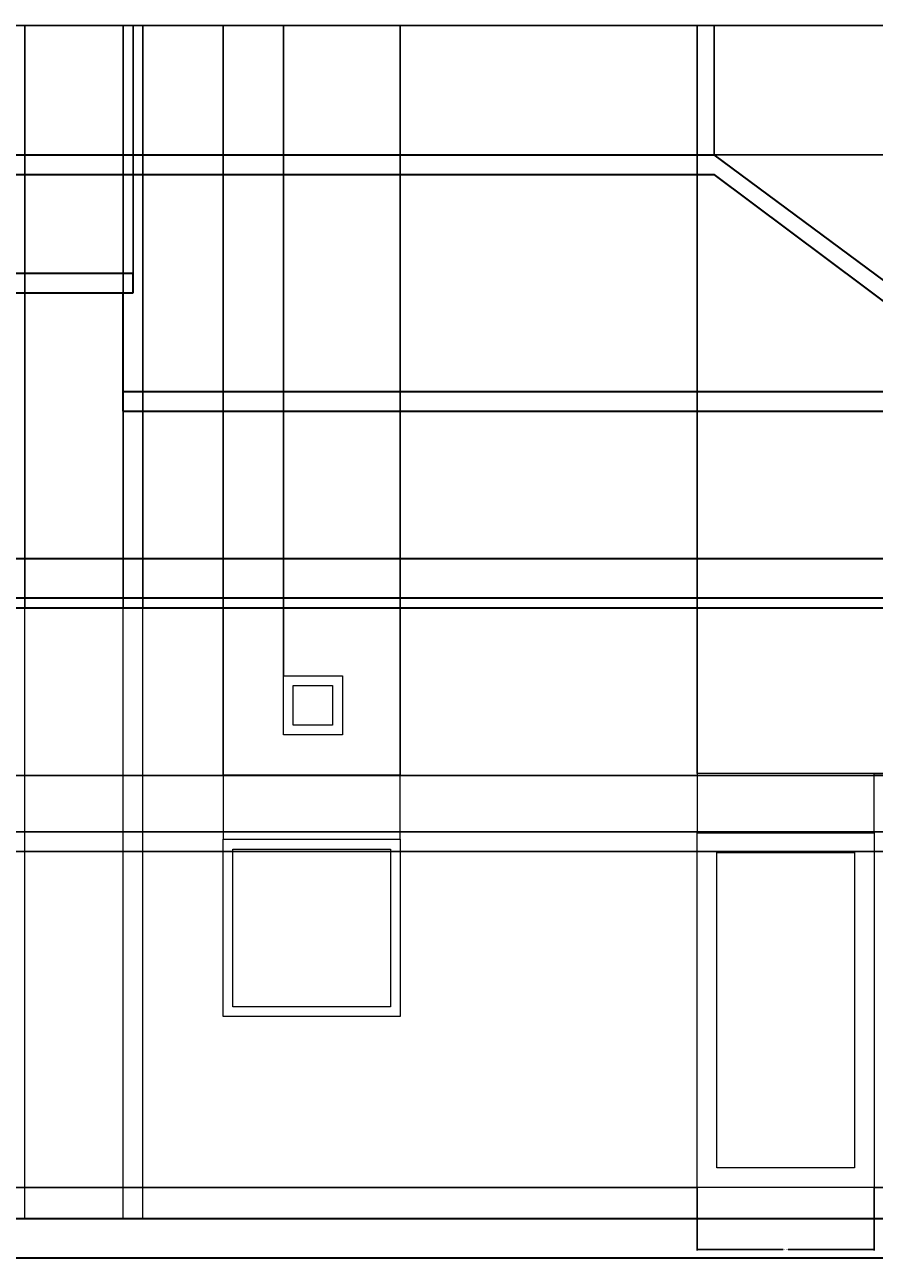
# Model space of a CAD drawing. Units: inches. Extents: x 1817 to 2378, y 1915 to 2370.
# Tile 5 of 8: x 1987 to 2160, y 2119 to 2370. Entities that reach past the tile are written whole.
import ezdxf

# ---------------------------------------------------------------- set-up
doc = ezdxf.new("R2010")
doc.units = ezdxf.units.IN
for name, color, linetype, lineweight in [('A-ANNO-DIMS', 2, 'Continuous', 18), ('A-ELEV', 7, 'Continuous', 35), ('A-GLAZ', 4, 'Continuous', 18), ('P-PIPE', 6, 'Continuous', 18)]:
    doc.layers.add(name, color=color, linetype=linetype, lineweight=lineweight)
doc.styles.get("Standard").update_dxf_attribs({"font": 'arial.ttf'})
doc.dimstyles.get("Standard").update_dxf_attribs({"dimtxt": 0.18, "dimasz": 0.18, "dimexe": 0.18, "dimexo": 0.0625, "dimgap": 0.09, "dimtad": 0, "dimtih": 1, "dimtoh": 1, "dimdec": 4, "dimzin": 0, "dimdsep": 46, "dimtxsty": 'Standard', "dimcen": 0.09, "dimadec": 0, "dimazin": 0, "dimtfac": 1, "dimtdec": 4, "dimtofl": 0, "dimtmove": 0, "dimatfit": 3, "dimfxl": 1, "dimtolj": 1, "dimtzin": 0, "dimarcsym": 0})

# ---------------------------------------------------------------- blocks, each defined once
blk = doc.blocks.new('WIN-SQ-900')
for points in [[(1924.43, 2204.58), (1960.43, 2204.58), (1960.43, 2217.58), (1924.43, 2217.58)], [(1924.43, 2204.58), (1960.43, 2204.58), (1960.43, 2168.58), (1924.43, 2168.58)], [(1926.43, 2202.58), (1958.43, 2202.58), (1958.43, 2170.58), (1926.43, 2170.58)]]:
    blk.add_lwpolyline(points, close=True)
blk = doc.blocks.new('WIN-TALL-900')
for points in [[(2123.62, 2205.9), (2159.62, 2205.9), (2159.62, 2217.9), (2123.62, 2217.9)], [(2123.62, 2205.9), (2159.62, 2205.9), (2159.62, 2133.9), (2123.62, 2133.9)], [(2127.62, 2201.9), (2155.62, 2201.9), (2155.62, 2137.9), (2127.62, 2137.9)]]:
    blk.add_lwpolyline(points, close=True)
blk = doc.blocks.new('VENT-300')
for points in [[(1936.66, 2237.16), (1948.66, 2237.16), (1948.66, 2225.16), (1936.66, 2225.16)], [(1938.66, 2235.16), (1946.66, 2235.16), (1946.66, 2227.16), (1938.66, 2227.16)]]:
    blk.add_lwpolyline(points, close=True)
blk = doc.blocks.new('*D8')
at = {"layer": 'A-ANNO-DIMS', "color": 0, "lineweight": -2, "transparency": 16777216}
for p, q in [((2159.68, 2217.9), (2172.4, 2217.9)), ((2172.22, 2217.72), (2172.22, 2176.08)), ((2172.22, 2134.08), (2172.22, 2175.71)), ((2159.68, 2133.9), (2172.4, 2133.9))]:
    blk.add_line(p, q, dxfattribs=at)
at = {"layer": 'A-ANNO-DIMS', "color": 0, "transparency": 16777216}
for points in [[(2172.19, 2217.72), (2172.25, 2217.72), (2172.22, 2217.9)], [(2172.19, 2134.08), (2172.25, 2134.08), (2172.22, 2133.9)]]:
    blk.add_solid(points, dxfattribs=at)
at = {"layer": 'Defpoints', "color": 0, "transparency": 16777216}
for p in [(2159.62, 2217.9), (2172.22, 2217.9), (2159.62, 2133.9)]:
    blk.add_point(p, dxfattribs=at)
at = {"layer": 'A-ANNO-DIMS', "color": 0, "transparency": 16777216, "insert": (2172.22, 2175.9), "char_height": 0.18, "attachment_point": 5}
blk.add_mtext('\\A1;TALL WINDOW 84 TYP.', dxfattribs=at)
blk = doc.blocks.new('*D9')
at = {"layer": 'A-ANNO-DIMS', "color": 0, "lineweight": -2, "transparency": 16777216}
for p, q in [((2123.62, 2133.83), (2123.62, 2121.12)), ((2159.62, 2133.83), (2159.62, 2121.12)), ((2123.8, 2121.3), (2141.09, 2121.3)), ((2159.44, 2121.3), (2142.15, 2121.3))]:
    blk.add_line(p, q, dxfattribs=at)
at = {"layer": 'A-ANNO-DIMS', "color": 0, "transparency": 16777216}
for points in [[(2123.8, 2121.33), (2123.8, 2121.27), (2123.62, 2121.3)], [(2159.44, 2121.33), (2159.44, 2121.27), (2159.62, 2121.3)]]:
    blk.add_solid(points, dxfattribs=at)
at = {"layer": 'Defpoints', "color": 0, "transparency": 16777216}
for p in [(2123.62, 2133.9), (2159.62, 2133.9), (2159.62, 2121.3)]:
    blk.add_point(p, dxfattribs=at)
at = {"layer": 'A-ANNO-DIMS', "color": 0, "transparency": 16777216, "insert": (2141.62, 2121.3), "char_height": 0.18, "attachment_point": 5}
blk.add_mtext('\\A1;36 TYP.', dxfattribs=at)
blk = doc.blocks.new('*D23')
at = {"layer": 'A-ANNO-DIMS', "color": 0, "lineweight": -2, "transparency": 16777216}
for p, q in [((2320.11, 2156.45), (2320.11, 1915.08)), ((1867.08, 1965.45), (1867.08, 1915.08)), ((1867.26, 1915.26), (2093.3, 1915.26)), ((2319.93, 1915.26), (2093.89, 1915.26))]:
    blk.add_line(p, q, dxfattribs=at)
at = {"layer": 'A-ANNO-DIMS', "color": 0, "transparency": 16777216}
for points in [[(1867.26, 1915.29), (1867.26, 1915.23), (1867.08, 1915.26)], [(2319.93, 1915.29), (2319.93, 1915.23), (2320.11, 1915.26)]]:
    blk.add_solid(points, dxfattribs=at)
at = {"layer": 'Defpoints', "color": 0, "transparency": 16777216}
for p in [(2320.11, 2156.51), (1867.08, 1965.51), (2320.11, 1915.26)]:
    blk.add_point(p, dxfattribs=at)
at = {"layer": 'A-ANNO-DIMS', "color": 0, "transparency": 16777216, "insert": (2093.6, 1915.26), "char_height": 0.18, "attachment_point": 5}
blk.add_mtext('\\A1;453', dxfattribs=at)
blk = doc.blocks.new('*D30')
at = {"layer": 'A-ANNO-DIMS', "color": 0, "lineweight": -2, "transparency": 16777216}
for p, q in [((1987.08, 2251.57), (1987.08, 2369.94)), ((1987.26, 2369.76), (1996.86, 2369.76)), ((2006.9, 2369.76), (1997.31, 2369.76)), ((2007.08, 2251.57), (2007.08, 2369.94))]:
    blk.add_line(p, q, dxfattribs=at)
at = {"layer": 'A-ANNO-DIMS', "color": 0, "transparency": 16777216}
for points in [[(1987.26, 2369.79), (1987.26, 2369.73), (1987.08, 2369.76)], [(2006.9, 2369.79), (2006.9, 2369.73), (2007.08, 2369.76)]]:
    blk.add_solid(points, dxfattribs=at)
at = {"layer": 'Defpoints', "color": 0, "transparency": 16777216}
for p in [(2007.08, 2369.76), (1987.08, 2251.51), (2007.08, 2251.51)]:
    blk.add_point(p, dxfattribs=at)
at = {"layer": 'A-ANNO-DIMS', "color": 0, "transparency": 16777216, "insert": (1997.08, 2369.76), "char_height": 0.18, "attachment_point": 5}
blk.add_mtext('\\A1;20', dxfattribs=at)
blk = doc.blocks.new('*D31')
at = {"layer": 'A-ANNO-DIMS', "color": 0, "lineweight": -2, "transparency": 16777216}
for p, q in [((2007.08, 2251.57), (2007.08, 2369.94)), ((2007.26, 2369.76), (2008.93, 2369.76)), ((2010.9, 2369.76), (2009.24, 2369.76)), ((2011.08, 2251.57), (2011.08, 2369.94))]:
    blk.add_line(p, q, dxfattribs=at)
at = {"layer": 'A-ANNO-DIMS', "color": 0, "transparency": 16777216}
for points in [[(2007.26, 2369.79), (2007.26, 2369.73), (2007.08, 2369.76)], [(2010.9, 2369.79), (2010.9, 2369.73), (2011.08, 2369.76)]]:
    blk.add_solid(points, dxfattribs=at)
at = {"layer": 'Defpoints', "color": 0, "transparency": 16777216}
for p in [(2011.08, 2369.76), (2007.08, 2251.51), (2011.08, 2251.51)]:
    blk.add_point(p, dxfattribs=at)
at = {"layer": 'A-ANNO-DIMS', "color": 0, "transparency": 16777216, "insert": (2009.08, 2369.76), "char_height": 0.18, "attachment_point": 5}
blk.add_mtext('\\A1;4', dxfattribs=at)
blk = doc.blocks.new('*D32')
at = {"layer": 'A-ANNO-DIMS', "color": 0, "lineweight": -2, "transparency": 16777216}
for p, q in [((2011.08, 2251.57), (2011.08, 2369.94)), ((2011.26, 2369.76), (2018.83, 2369.76)), ((2027.17, 2369.76), (2019.61, 2369.76)), ((2027.35, 2217.64), (2027.35, 2369.94))]:
    blk.add_line(p, q, dxfattribs=at)
at = {"layer": 'A-ANNO-DIMS', "color": 0, "transparency": 16777216}
for points in [[(2011.26, 2369.79), (2011.26, 2369.73), (2011.08, 2369.76)], [(2027.17, 2369.79), (2027.17, 2369.73), (2027.35, 2369.76)]]:
    blk.add_solid(points, dxfattribs=at)
at = {"layer": 'Defpoints', "color": 0, "transparency": 16777216}
for p in [(2027.35, 2369.76), (2011.08, 2251.51), (2027.35, 2217.58)]:
    blk.add_point(p, dxfattribs=at)
at = {"layer": 'A-ANNO-DIMS', "color": 0, "transparency": 16777216, "insert": (2019.22, 2369.76), "char_height": 0.18, "attachment_point": 5}
blk.add_mtext('\\A1;16.27', dxfattribs=at)
blk = doc.blocks.new('*D33')
at = {"layer": 'A-ANNO-DIMS', "color": 0, "lineweight": -2, "transparency": 16777216}
for p, q in [((2027.35, 2217.64), (2027.35, 2369.94)), ((2027.53, 2369.76), (2033.03, 2369.76)), ((2039.43, 2369.76), (2033.94, 2369.76)), ((2039.61, 2237.83), (2039.61, 2369.94))]:
    blk.add_line(p, q, dxfattribs=at)
at = {"layer": 'A-ANNO-DIMS', "color": 0, "transparency": 16777216}
for points in [[(2027.53, 2369.79), (2027.53, 2369.73), (2027.35, 2369.76)], [(2039.43, 2369.79), (2039.43, 2369.73), (2039.61, 2369.76)]]:
    blk.add_solid(points, dxfattribs=at)
at = {"layer": 'Defpoints', "color": 0, "transparency": 16777216}
for p in [(2039.61, 2369.76), (2039.61, 2237.77), (2027.35, 2217.58)]:
    blk.add_point(p, dxfattribs=at)
at = {"layer": 'A-ANNO-DIMS', "color": 0, "transparency": 16777216, "insert": (2033.48, 2369.76), "char_height": 0.18, "attachment_point": 5}
blk.add_mtext('\\A1;12.256', dxfattribs=at)
blk = doc.blocks.new('*D34')
at = {"layer": 'A-ANNO-DIMS', "color": 0, "lineweight": -2, "transparency": 16777216}
for p, q in [((2039.61, 2237.83), (2039.61, 2369.94)), ((2039.79, 2369.76), (2051.02, 2369.76)), ((2063.17, 2369.76), (2051.95, 2369.76)), ((2063.35, 2217.64), (2063.35, 2369.94))]:
    blk.add_line(p, q, dxfattribs=at)
at = {"layer": 'A-ANNO-DIMS', "color": 0, "transparency": 16777216}
for points in [[(2039.79, 2369.79), (2039.79, 2369.73), (2039.61, 2369.76)], [(2063.17, 2369.79), (2063.17, 2369.73), (2063.35, 2369.76)]]:
    blk.add_solid(points, dxfattribs=at)
at = {"layer": 'Defpoints', "color": 0, "transparency": 16777216}
for p in [(2063.35, 2369.76), (2039.61, 2237.77), (2063.35, 2217.58)]:
    blk.add_point(p, dxfattribs=at)
at = {"layer": 'A-ANNO-DIMS', "color": 0, "transparency": 16777216, "insert": (2051.48, 2369.76), "char_height": 0.18, "attachment_point": 5}
blk.add_mtext('\\A1;23.744', dxfattribs=at)
blk = doc.blocks.new('*D35')
at = {"layer": 'A-ANNO-DIMS', "color": 0, "lineweight": -2, "transparency": 16777216}
for p, q in [((2063.35, 2217.64), (2063.35, 2369.94)), ((2063.53, 2369.76), (2093.09, 2369.76)), ((2123.44, 2369.76), (2093.88, 2369.76)), ((2123.62, 2217.96), (2123.62, 2369.94))]:
    blk.add_line(p, q, dxfattribs=at)
at = {"layer": 'A-ANNO-DIMS', "color": 0, "transparency": 16777216}
for points in [[(2063.53, 2369.79), (2063.53, 2369.73), (2063.35, 2369.76)], [(2123.44, 2369.79), (2123.44, 2369.73), (2123.62, 2369.76)]]:
    blk.add_solid(points, dxfattribs=at)
at = {"layer": 'Defpoints', "color": 0, "transparency": 16777216}
for p in [(2123.62, 2369.76), (2123.62, 2217.9), (2063.35, 2217.58)]:
    blk.add_point(p, dxfattribs=at)
at = {"layer": 'A-ANNO-DIMS', "color": 0, "transparency": 16777216, "insert": (2093.49, 2369.76), "char_height": 0.18, "attachment_point": 5}
blk.add_mtext('\\A1;60.26', dxfattribs=at)
blk = doc.blocks.new('*D44')
at = {"layer": 'A-ANNO-DIMS', "color": 0, "lineweight": -2, "transparency": 16777216}
for p, q in [((1903.08, 2261.57), (1903.08, 2369.94)), ((1903.26, 2369.76), (1954.8, 2369.76)), ((2006.9, 2369.76), (1955.36, 2369.76)), ((2007.08, 2291.57), (2007.08, 2369.94))]:
    blk.add_line(p, q, dxfattribs=at)
at = {"layer": 'A-ANNO-DIMS', "color": 0, "transparency": 16777216}
for points in [[(1903.26, 2369.79), (1903.26, 2369.73), (1903.08, 2369.76)], [(2006.9, 2369.79), (2006.9, 2369.73), (2007.08, 2369.76)]]:
    blk.add_solid(points, dxfattribs=at)
at = {"layer": 'Defpoints', "color": 0, "transparency": 16777216}
for p in [(2007.08, 2369.76), (2007.08, 2291.51), (1903.08, 2261.51)]:
    blk.add_point(p, dxfattribs=at)
at = {"layer": 'A-ANNO-DIMS', "color": 0, "transparency": 16777216, "insert": (1955.08, 2369.76), "char_height": 0.18, "attachment_point": 5}
blk.add_mtext('\\A1;104', dxfattribs=at)
blk = doc.blocks.new('*D45')
at = {"layer": 'A-ANNO-DIMS', "color": 0, "lineweight": -2, "transparency": 16777216}
for p, q in [((2007.08, 2291.57), (2007.08, 2369.94)), ((2007.26, 2369.76), (2007.94, 2369.76)), ((2008.9, 2369.76), (2008.23, 2369.76)), ((2009.08, 2319.57), (2009.08, 2369.94))]:
    blk.add_line(p, q, dxfattribs=at)
at = {"layer": 'A-ANNO-DIMS', "color": 0, "transparency": 16777216}
for points in [[(2007.26, 2369.79), (2007.26, 2369.73), (2007.08, 2369.76)], [(2008.9, 2369.79), (2008.9, 2369.73), (2009.08, 2369.76)]]:
    blk.add_solid(points, dxfattribs=at)
at = {"layer": 'Defpoints', "color": 0, "transparency": 16777216}
for p in [(2009.08, 2369.76), (2009.08, 2319.51), (2007.08, 2291.51)]:
    blk.add_point(p, dxfattribs=at)
at = {"layer": 'A-ANNO-DIMS', "color": 0, "transparency": 16777216, "insert": (2008.08, 2369.76), "char_height": 0.18, "attachment_point": 5}
blk.add_mtext('\\A1;2', dxfattribs=at)
blk = doc.blocks.new('*D46')
at = {"layer": 'A-ANNO-DIMS', "color": 0, "lineweight": -2, "transparency": 16777216}
for p, q in [((2009.08, 2319.57), (2009.08, 2369.94)), ((2009.26, 2369.76), (2067.8, 2369.76)), ((2126.9, 2369.76), (2068.37, 2369.76)), ((2127.08, 2343.57), (2127.08, 2369.94))]:
    blk.add_line(p, q, dxfattribs=at)
at = {"layer": 'A-ANNO-DIMS', "color": 0, "transparency": 16777216}
for points in [[(2009.26, 2369.79), (2009.26, 2369.73), (2009.08, 2369.76)], [(2126.9, 2369.79), (2126.9, 2369.73), (2127.08, 2369.76)]]:
    blk.add_solid(points, dxfattribs=at)
at = {"layer": 'Defpoints', "color": 0, "transparency": 16777216}
for p in [(2127.08, 2369.76), (2127.08, 2343.51), (2009.08, 2319.51)]:
    blk.add_point(p, dxfattribs=at)
at = {"layer": 'A-ANNO-DIMS', "color": 0, "transparency": 16777216, "insert": (2068.08, 2369.76), "char_height": 0.18, "attachment_point": 5}
blk.add_mtext('\\A1;118', dxfattribs=at)
blk = doc.blocks.new('*D47')
at = {"layer": 'A-ANNO-DIMS', "color": 0, "lineweight": -2, "transparency": 16777216}
for p, q in [((2127.08, 2343.57), (2127.08, 2369.94)), ((2127.26, 2369.76), (2159.09, 2369.76)), ((2191.7, 2369.76), (2159.87, 2369.76)), ((2191.88, 2295.57), (2191.88, 2369.94))]:
    blk.add_line(p, q, dxfattribs=at)
at = {"layer": 'A-ANNO-DIMS', "color": 0, "transparency": 16777216}
for points in [[(2127.26, 2369.79), (2127.26, 2369.73), (2127.08, 2369.76)], [(2191.7, 2369.79), (2191.7, 2369.73), (2191.88, 2369.76)]]:
    blk.add_solid(points, dxfattribs=at)
at = {"layer": 'Defpoints', "color": 0, "transparency": 16777216}
for p in [(2191.88, 2369.76), (2127.08, 2343.51), (2191.88, 2295.51)]:
    blk.add_point(p, dxfattribs=at)
at = {"layer": 'A-ANNO-DIMS', "color": 0, "transparency": 16777216, "insert": (2159.48, 2369.76), "char_height": 0.18, "attachment_point": 5}
blk.add_mtext('\\A1;64.79', dxfattribs=at)
blk = doc.blocks.new('*D51')
at = {"layer": 'A-ANNO-DIMS', "color": 0, "lineweight": -2, "transparency": 16777216}
for p, q in [((2281.02, 2261.51), (1817.4, 2261.51)), ((1817.58, 2261.33), (1817.58, 2257.69)), ((1817.58, 2253.69), (1817.58, 2257.33)), ((2289.54, 2253.51), (1817.4, 2253.51))]:
    blk.add_line(p, q, dxfattribs=at)
at = {"layer": 'A-ANNO-DIMS', "color": 0, "transparency": 16777216}
for points in [[(1817.55, 2261.33), (1817.61, 2261.33), (1817.58, 2261.51)], [(1817.55, 2253.69), (1817.61, 2253.69), (1817.58, 2253.51)]]:
    blk.add_solid(points, dxfattribs=at)
at = {"layer": 'Defpoints', "color": 0, "transparency": 16777216}
for p in [(1817.58, 2261.51), (2281.08, 2261.51), (2289.61, 2253.51)]:
    blk.add_point(p, dxfattribs=at)
at = {"layer": 'A-ANNO-DIMS', "color": 0, "transparency": 16777216, "insert": (1817.58, 2257.51), "char_height": 0.18, "attachment_point": 5}
blk.add_mtext('\\A1;8', dxfattribs=at)
blk = doc.blocks.new('*D79')
at = {"layer": 'A-ANNO-DIMS', "color": 0, "lineweight": -2, "transparency": 16777216}
for p, q in [((2127.15, 2343.51), (2377.4, 2343.51)), ((2377.22, 2343.33), (2377.22, 2319.69)), ((2377.22, 2295.69), (2377.22, 2319.33)), ((2283.15, 2295.51), (2377.4, 2295.51))]:
    blk.add_line(p, q, dxfattribs=at)
at = {"layer": 'A-ANNO-DIMS', "color": 0, "transparency": 16777216}
for points in [[(2377.19, 2343.33), (2377.25, 2343.33), (2377.22, 2343.51)], [(2377.19, 2295.69), (2377.25, 2295.69), (2377.22, 2295.51)]]:
    blk.add_solid(points, dxfattribs=at)
at = {"layer": 'Defpoints', "color": 0, "transparency": 16777216}
for p in [(2127.08, 2343.51), (2377.22, 2343.51), (2283.08, 2295.51)]:
    blk.add_point(p, dxfattribs=at)
at = {"layer": 'A-ANNO-DIMS', "color": 0, "transparency": 16777216, "insert": (2377.22, 2319.51), "char_height": 0.18, "attachment_point": 5}
blk.add_mtext('\\A1;48', dxfattribs=at)
blk = doc.blocks.new('*D82')
at = {"layer": 'A-ANNO-DIMS', "color": 0, "lineweight": -2, "transparency": 16777216}
for p, q in [((2123.56, 2133.9), (1817.4, 2133.9)), ((1817.58, 2133.72), (1817.58, 2130.88)), ((1817.58, 2127.69), (1817.58, 2130.52)), ((2198.53, 2127.51), (1817.4, 2127.51))]:
    blk.add_line(p, q, dxfattribs=at)
at = {"layer": 'A-ANNO-DIMS', "color": 0, "transparency": 16777216}
for points in [[(1817.55, 2133.72), (1817.61, 2133.72), (1817.58, 2133.9)], [(1817.55, 2127.69), (1817.61, 2127.69), (1817.58, 2127.51)]]:
    blk.add_solid(points, dxfattribs=at)
at = {"layer": 'Defpoints', "color": 0, "transparency": 16777216}
for p in [(1817.58, 2133.9), (2123.62, 2133.9), (2198.59, 2127.51)]:
    blk.add_point(p, dxfattribs=at)
at = {"layer": 'A-ANNO-DIMS', "color": 0, "transparency": 16777216, "insert": (1817.58, 2130.7), "char_height": 0.18, "attachment_point": 5}
blk.add_mtext('\\A1;6.387', dxfattribs=at)
blk = doc.blocks.new('*D104')
at = {"layer": 'A-ANNO-DIMS', "color": 0, "lineweight": -2, "transparency": 16777216}
for p, q in [((2210.55, 2217.51), (1817.4, 2217.51)), ((1817.58, 2217.33), (1817.58, 2211.97)), ((1817.58, 2206.26), (1817.58, 2211.61)), ((2210.55, 2206.08), (1817.4, 2206.08))]:
    blk.add_line(p, q, dxfattribs=at)
at = {"layer": 'A-ANNO-DIMS', "color": 0, "transparency": 16777216}
for points in [[(1817.55, 2217.33), (1817.61, 2217.33), (1817.58, 2217.51)], [(1817.55, 2206.26), (1817.61, 2206.26), (1817.58, 2206.08)]]:
    blk.add_solid(points, dxfattribs=at)
at = {"layer": 'Defpoints', "color": 0, "transparency": 16777216}
for p in [(2210.62, 2217.51), (1817.58, 2206.08), (2210.62, 2206.08)]:
    blk.add_point(p, dxfattribs=at)
at = {"layer": 'A-ANNO-DIMS', "color": 0, "transparency": 16777216, "insert": (1817.58, 2211.79), "char_height": 0.18, "attachment_point": 5}
blk.add_mtext('\\A1;11.433', dxfattribs=at)
blk = doc.blocks.new('*D105')
at = {"layer": 'A-ANNO-DIMS', "color": 0, "lineweight": -2, "transparency": 16777216}
for p, q in [((2210.55, 2206.08), (1817.4, 2206.08)), ((1817.58, 2205.9), (1817.58, 2204.26)), ((1817.58, 2202.26), (1817.58, 2203.89)), ((2214.55, 2202.08), (1817.4, 2202.08))]:
    blk.add_line(p, q, dxfattribs=at)
at = {"layer": 'A-ANNO-DIMS', "color": 0, "transparency": 16777216}
for points in [[(1817.55, 2205.9), (1817.61, 2205.9), (1817.58, 2206.08)], [(1817.55, 2202.26), (1817.61, 2202.26), (1817.58, 2202.08)]]:
    blk.add_solid(points, dxfattribs=at)
at = {"layer": 'Defpoints', "color": 0, "transparency": 16777216}
for p in [(2210.62, 2206.08), (1817.58, 2202.08), (2214.62, 2202.08)]:
    blk.add_point(p, dxfattribs=at)
at = {"layer": 'A-ANNO-DIMS', "color": 0, "transparency": 16777216, "insert": (1817.58, 2204.08), "char_height": 0.18, "attachment_point": 5}
blk.add_mtext('\\A1;4.00', dxfattribs=at)
blk = doc.blocks.new('*D119')
at = {"layer": 'A-ANNO-DIMS', "color": 0, "lineweight": -2, "transparency": 16777216}
for p, q in [((1903.08, 1989.57), (1903.08, 2369.94)), ((1903.26, 2369.76), (2091.62, 2369.76)), ((2280.9, 2369.76), (2092.55, 2369.76)), ((2281.08, 1989.57), (2281.08, 2369.94))]:
    blk.add_line(p, q, dxfattribs=at)
at = {"layer": 'A-ANNO-DIMS', "color": 0, "transparency": 16777216}
for points in [[(1903.26, 2369.79), (1903.26, 2369.73), (1903.08, 2369.76)], [(2280.9, 2369.79), (2280.9, 2369.73), (2281.08, 2369.76)]]:
    blk.add_solid(points, dxfattribs=at)
at = {"layer": 'Defpoints', "color": 0, "transparency": 16777216}
for p in [(2281.08, 2369.76), (1903.08, 1989.51), (2281.08, 1989.51)]:
    blk.add_point(p, dxfattribs=at)
at = {"layer": 'A-ANNO-DIMS', "color": 0, "transparency": 16777216, "insert": (2092.08, 2369.76), "char_height": 0.18, "attachment_point": 5}
blk.add_mtext('\\A1;378.00', dxfattribs=at)

msp = doc.modelspace()

# ---------------------------------------------------------------- linework, layer by layer
at = {"layer": 'A-ELEV'}
for p, q in [((1901.0849, 2343.5087), (2127.0849, 2343.5087)), ((2191.8757, 2295.5087), (2127.0849, 2343.5087)), ((1901.0849, 2339.5087), (2127.0849, 2339.5087)), ((2186.0507, 2295.5087), (2127.0849, 2339.5087)), ((1901.0849, 2319.5087), (2009.0849, 2319.5087)), ((2009.0849, 2315.5087), (2009.0849, 2319.5087)), ((1901.0849, 2315.5087), (2009.0849, 2315.5087)), ((2007.0849, 2291.5087), (2007.0849, 2315.5087)), ((2007.0849, 2295.5087), (2283.0849, 2295.5087)), ((2007.0849, 2291.5087), (2283.0849, 2291.5087)), ((2281.0849, 2261.5087), (1903.0849, 2261.5087)), ((2289.6055, 2253.5087), (1894.506, 2253.5087)), ((2289.6055, 2251.5087), (1894.506, 2251.5087)), ((2198.5896, 2127.5087), (1903.0849, 2127.5087)), ((2198.5896, 2119.5087), (1895.6961, 2119.5087))]:
    msp.add_line(p, q, dxfattribs=at)
at = {"layer": 'P-PIPE'}
for p, q in [((1987.0849, 2127.5087), (1987.0849, 2251.5087)), ((2007.0849, 2127.5087), (2007.0849, 2251.5087)), ((2011.0849, 2127.5087), (2011.0849, 2251.5087))]:
    msp.add_line(p, q, dxfattribs=at)

# ---------------------------------------------------------------- block references
at = {"layer": 'A-GLAZ'}
for name, p in [('VENT-300', (102.9456, 0.6122)), ('WIN-TALL-900', (0, 0)), ('WIN-SQ-900', (102.9291, 0))]:
    msp.add_blockref(name, p, dxfattribs=at)

# ---------------------------------------------------------------- dimensions: what is measured, and where the dimension line sits
at = {"layer": 'A-ANNO-DIMS'}
for base, p1, p2, override, picture, middle in [((2007.0849, 2369.7587), (1903.0849, 2261.5087), (2007.0849, 2291.5087), {"dimdec": 0, "dimlfac": 1, "dimrnd": 0, "dimzin": 0, "dimdsep": 46, "dimlunit": 2}, '*D44', (1955.0849, 2369.7587)), ((2281.0849, 2369.7587), (1903.0849, 1989.5087), (2281.0849, 1989.5087), {"dimdec": 2, "dimlfac": 1, "dimrnd": 0, "dimzin": 0, "dimdsep": 46, "dimlunit": 2}, '*D119', (2092.0849, 2369.7587)), ((2007.0849, 2369.7587), (1987.0849, 2251.5087), (2007.0849, 2251.5087), {"dimdec": 0, "dimlfac": 1, "dimrnd": 0, "dimzin": 0, "dimdsep": 46, "dimlunit": 2}, '*D30', (1997.0849, 2369.7587)), ((2011.0849, 2369.7587), (2007.0849, 2251.5087), (2011.0849, 2251.5087), {"dimdec": 0, "dimlfac": 1, "dimrnd": 0, "dimzin": 0, "dimdsep": 46, "dimlunit": 2}, '*D31', (2009.0849, 2369.7587)), ((2009.0849, 2369.7587), (2007.0849, 2291.5087), (2009.0849, 2319.5087), {"dimdec": 0, "dimlfac": 1, "dimrnd": 0, "dimzin": 0, "dimdsep": 46, "dimlunit": 2}, '*D45', (2008.0849, 2369.7587)), ((2127.0849, 2369.7587), (2009.0849, 2319.5087), (2127.0849, 2343.5087), {"dimdec": 0, "dimlfac": 1, "dimrnd": 0, "dimzin": 0, "dimdsep": 46, "dimlunit": 2}, '*D46', (2068.0849, 2369.7587)), ((2027.3548, 2369.7587), (2011.0849, 2251.5087), (2027.3548, 2217.5813), {"dimdec": 2, "dimlfac": 1, "dimrnd": 0, "dimzin": 0, "dimdsep": 46, "dimlunit": 2}, '*D32', (2019.2199, 2369.7587)), ((2039.6105, 2369.7587), (2027.3548, 2217.5813), (2039.6105, 2237.7713), {"dimdec": 3, "dimlfac": 1, "dimrnd": 0, "dimzin": 0, "dimdsep": 46, "dimlunit": 2}, '*D33', (2033.4827, 2369.7587)), ((2063.3548, 2369.7587), (2039.6105, 2237.7713), (2063.3548, 2217.5813), {"dimdec": 3, "dimlfac": 1, "dimrnd": 0, "dimzin": 0, "dimdsep": 46, "dimlunit": 2}, '*D34', (2051.4827, 2369.7587)), ((2123.6179, 2369.7587), (2063.3548, 2217.5813), (2123.6179, 2217.8955), {"dimdec": 2, "dimlfac": 1, "dimrnd": 0, "dimzin": 0, "dimdsep": 46, "dimlunit": 2}, '*D35', (2093.4864, 2369.7587)), ((2191.8757, 2369.7587), (2127.0849, 2343.5087), (2191.8757, 2295.5087), {"dimdec": 2, "dimlfac": 1, "dimrnd": 0, "dimzin": 0, "dimdsep": 46, "dimlunit": 2}, '*D47', (2159.4803, 2369.7587)), ((2320.1054, 1915.2587), (1867.0849, 1965.5087), (2320.1054, 2156.5133), {"dimdec": 0, "dimlfac": 1, "dimrnd": 0, "dimzin": 0, "dimdsep": 46, "dimlunit": 2}, '*D23', (2093.5951, 1915.2587))]:
    dim = msp.add_linear_dim(base=base, p1=p1, p2=p2, dimstyle='Standard', override=override, dxfattribs=at)
    dim.commit()
    dim.dimension.update_dxf_attribs({"geometry": picture, "text_midpoint": middle})
for base, p1, p2, override, picture, middle in [((2377.2181, 2343.5087), (2283.0849, 2295.5087), (2127.0849, 2343.5087), {"dimdec": 0, "dimlfac": 1, "dimrnd": 0, "dimzin": 0, "dimdsep": 46, "dimlunit": 2}, '*D79', (2377.2181, 2319.5087)), ((1817.584, 2261.5087), (2289.6055, 2253.5087), (2281.0849, 2261.5087), {"dimdec": 0, "dimlfac": 1, "dimrnd": 0, "dimzin": 0, "dimdsep": 46, "dimlunit": 2}, '*D51', (1817.584, 2257.5087)), ((1817.584, 2206.0753), (2210.6163, 2217.5087), (2210.6163, 2206.0753), {"dimdec": 3, "dimlfac": 1, "dimrnd": 0, "dimzin": 0, "dimdsep": 46, "dimlunit": 2}, '*D104', (1817.584, 2211.792)), ((1817.584, 2202.0753), (2210.6163, 2206.0753), (2214.6163, 2202.0753), {"dimdec": 2, "dimlfac": 1, "dimrnd": 0, "dimzin": 0, "dimdsep": 46, "dimlunit": 2}, '*D105', (1817.584, 2204.0753)), ((1817.584, 2133.8955), (2198.5896, 2127.5087), (2123.6179, 2133.8955), {"dimdec": 3, "dimlfac": 1, "dimrnd": 0, "dimzin": 0, "dimdsep": 46, "dimlunit": 2}, '*D82', (1817.584, 2130.7021))]:
    dim = msp.add_linear_dim(base=base, p1=p1, p2=p2, angle=90, dimstyle='Standard', override=override, dxfattribs=at)
    dim.commit()
    dim.dimension.update_dxf_attribs({"geometry": picture, "text_midpoint": middle})
dim = msp.add_linear_dim(base=(2172.2179, 2217.8955), p1=(2159.6179, 2133.8955), p2=(2159.6179, 2217.8955), angle=90, text='TALL WINDOW <> TYP.', dimstyle='Standard', override={"dimdec": 0, "dimlfac": 1, "dimrnd": 0, "dimzin": 0, "dimdsep": 46, "dimlunit": 2}, dxfattribs=at)
dim.commit()
dim.dimension.update_dxf_attribs({"geometry": '*D8', "text_midpoint": (2172.2179, 2175.8955)})
dim = msp.add_linear_dim(base=(2159.6179, 2121.2955), p1=(2123.6179, 2133.8955), p2=(2159.6179, 2133.8955), text='<> TYP.', dimstyle='Standard', override={"dimdec": 0, "dimlfac": 1, "dimrnd": 0, "dimzin": 0, "dimdsep": 46, "dimlunit": 2}, dxfattribs=at)
dim.commit()
dim.dimension.update_dxf_attribs({"geometry": '*D9', "text_midpoint": (2141.6179, 2121.2955)})

doc.saveas('drawing.dxf')
